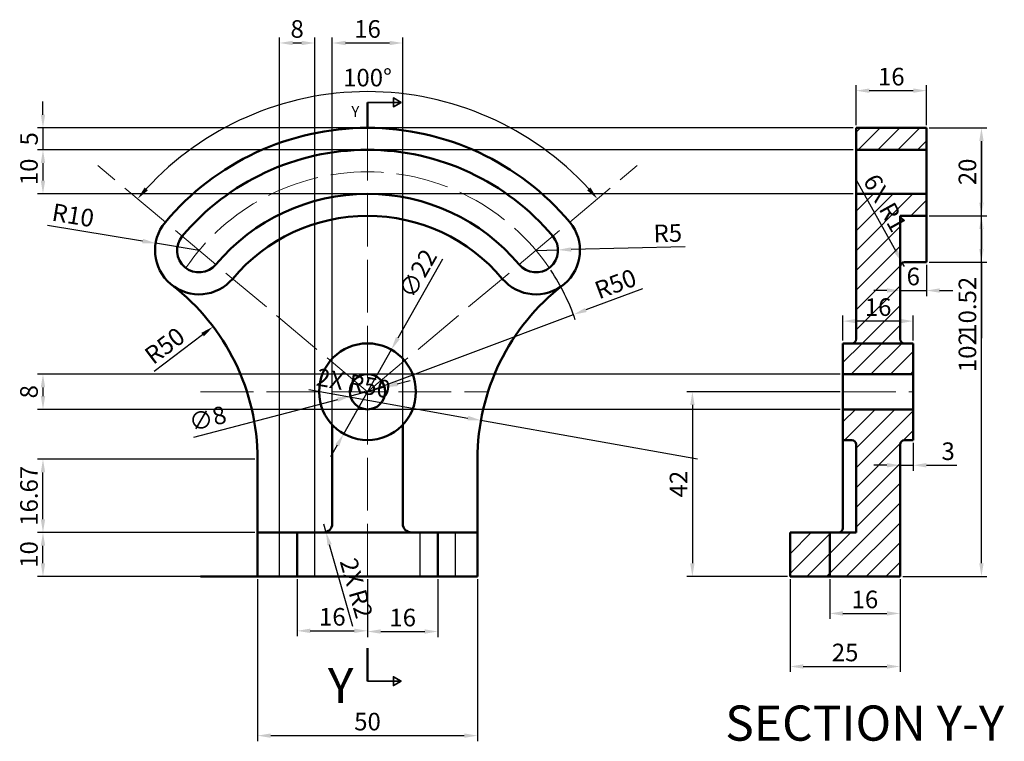
# Model space of a CAD drawing. Units: millimetres. Extents: x 867 to 1199, y -58 to 305.
# Tile 3 of 3: x 867 to 1091, y 141 to 305. Entities that reach past the tile are written whole.
import ezdxf

# ---------------------------------------------------------------- set-up
doc = ezdxf.new("R2010")
doc.units = ezdxf.units.MM
doc.linetypes.add('ACAD_ISO02W100', pattern=[15, 12, -3])
for name, color, linetype, lineweight in [('M-CNTR', 1, 'ACAD_ISO02W100', 18), ('M-DIMS', 2, 'Continuous', 25), ('M-HATC', 8, 'Continuous', 18), ('M-HIDN', 6, 'ACAD_ISO02W100', 25), ('M-OUTL', 7, 'Continuous', 50), ('M-SECT', 4, 'Continuous', 35), ('M-TEXT', 3, 'Continuous', 25)]:
    doc.layers.add(name, color=color, linetype=linetype, lineweight=lineweight)
doc.styles.get("Standard").update_dxf_attribs({"font": 'arial.ttf'})
doc.dimstyles.new('ISO-25', dxfattribs={"dimtxt": 4, "dimasz": 3, "dimexe": 1.25, "dimexo": 0.625, "dimtad": 1, "dimdec": 1, "dimtxsty": 'Standard', "dimcen": 2.5, "dimadec": 0, "dimazin": 0, "dimtfac": 1, "dimtdec": 1, "dimtmove": 0, "dimatfit": 3, "dimfxl": 1, "dimarcsym": 0})
pattern_1 = [(45, (-91.2894, -451.28), (-2.245064, 2.245064), [])]

# ---------------------------------------------------------------- blocks, each defined once
blk = doc.blocks.new('*D1')
at = {"layer": 'Defpoints', "color": 0, "transparency": 16777216}
for p in [(921.2, 178.7), (971.2, 178.7), (971.2, 142.51)]:
    blk.add_point(p, dxfattribs=at)
at = {"layer": 'M-DIMS', "color": 0, "lineweight": -2, "transparency": 16777216}
for p, q in [((921.2, 178.08), (921.2, 141.26)), ((971.2, 178.08), (971.2, 141.26)), ((924.2, 142.51), (968.2, 142.51))]:
    blk.add_line(p, q, dxfattribs=at)
at = {"layer": 'M-DIMS', "color": 0, "transparency": 16777216}
for points in [[(924.2, 143.01), (924.2, 142.01), (921.2, 142.51)], [(968.2, 143.01), (968.2, 142.01), (971.2, 142.51)]]:
    blk.add_solid(points, dxfattribs=at)
at = {"layer": 'M-DIMS', "color": 0, "transparency": 16777216, "insert": (946.2, 145.18), "char_height": 4, "attachment_point": 5}
blk.add_mtext('50', dxfattribs=at)
blk = doc.blocks.new('*D2')
at = {"layer": 'Defpoints', "color": 0, "transparency": 16777216}
for p in [(930.2, 178.7), (946.2, 178.7), (946.2, 166.34)]:
    blk.add_point(p, dxfattribs=at)
at = {"layer": 'M-DIMS', "color": 0, "lineweight": -2, "transparency": 16777216}
for p, q in [((930.2, 178.08), (930.2, 165.09)), ((946.2, 178.08), (946.2, 165.09)), ((933.2, 166.34), (943.2, 166.34))]:
    blk.add_line(p, q, dxfattribs=at)
at = {"layer": 'M-DIMS', "color": 0, "transparency": 16777216}
for points in [[(933.2, 166.84), (933.2, 165.84), (930.2, 166.34)], [(943.2, 166.84), (943.2, 165.84), (946.2, 166.34)]]:
    blk.add_solid(points, dxfattribs=at)
at = {"layer": 'M-DIMS', "color": 0, "transparency": 16777216, "insert": (938.2, 169.01), "char_height": 4, "attachment_point": 5}
blk.add_mtext('16', dxfattribs=at)
blk = doc.blocks.new('*D3')
at = {"layer": 'Defpoints', "color": 0, "transparency": 16777216}
for p in [(946.2, 178.7), (962.2, 178.7), (962.2, 166.18)]:
    blk.add_point(p, dxfattribs=at)
at = {"layer": 'M-DIMS', "color": 0, "lineweight": -2, "transparency": 16777216}
for p, q in [((946.2, 178.08), (946.2, 164.93)), ((962.2, 178.08), (962.2, 164.93)), ((949.2, 166.18), (959.2, 166.18))]:
    blk.add_line(p, q, dxfattribs=at)
at = {"layer": 'M-DIMS', "color": 0, "transparency": 16777216}
for points in [[(949.2, 166.68), (949.2, 165.68), (946.2, 166.18)], [(959.2, 166.68), (959.2, 165.68), (962.2, 166.18)]]:
    blk.add_solid(points, dxfattribs=at)
at = {"layer": 'M-DIMS', "color": 0, "transparency": 16777216, "insert": (954.2, 168.84), "char_height": 4, "attachment_point": 5}
blk.add_mtext('16', dxfattribs=at)
blk = doc.blocks.new('*D4')
at = {"layer": 'Defpoints', "color": 0, "transparency": 16777216}
for p in [(898.03, 254.48), (907.9, 252.84)]:
    blk.add_point(p, dxfattribs=at)
at = {"layer": 'M-DIMS', "color": 0, "lineweight": -2, "transparency": 16777216}
for p, q in [((873.42, 258.58), (895.07, 254.98)), ((907.9, 252.84), (898.03, 254.48))]:
    blk.add_line(p, q, dxfattribs=at)
at = {"layer": 'M-DIMS', "color": 0, "transparency": 16777216}
blk.add_solid([(895.16, 255.47), (894.99, 254.48), (898.03, 254.48)], dxfattribs=at)
at = {"layer": 'M-DIMS', "color": 0, "transparency": 16777216, "insert": (879.18, 260.33), "char_height": 4, "attachment_point": 5, "rotation": 350.5421}
blk.add_mtext('R10', dxfattribs=at)
blk = doc.blocks.new('*D5')
at = {"layer": 'Defpoints', "color": 0, "transparency": 16777216}
for p in [(989.5, 252.96), (984.5, 252.84)]:
    blk.add_point(p, dxfattribs=at)
at = {"layer": 'M-DIMS', "color": 0, "lineweight": -2, "transparency": 16777216}
for p, q in [((984.5, 252.84), (989.5, 252.96)), ((1018.41, 253.67), (992.5, 253.04))]:
    blk.add_line(p, q, dxfattribs=at)
at = {"layer": 'M-DIMS', "color": 0, "transparency": 16777216}
blk.add_solid([(992.49, 253.54), (992.51, 252.54), (989.5, 252.96)], dxfattribs=at)
at = {"layer": 'M-DIMS', "color": 0, "transparency": 16777216, "insert": (1014.48, 256.24), "char_height": 4, "attachment_point": 5, "rotation": 1.4057}
blk.add_mtext('R5', dxfattribs=at)
blk = doc.blocks.new('*D6')
at = {"layer": 'Defpoints', "color": 0, "transparency": 16777216}
for p in [(993.02, 238.24), (946.2, 220.7)]:
    blk.add_point(p, dxfattribs=at)
at = {"layer": 'M-DIMS', "color": 0, "lineweight": -2, "transparency": 16777216}
for p, q in [((1008.75, 244.13), (995.83, 239.29)), ((946.2, 220.7), (993.02, 238.24))]:
    blk.add_line(p, q, dxfattribs=at)
blk.add_arc((946.2, 220.7), 50, 19.1042, 33.5518, dxfattribs=at)
at = {"layer": 'M-DIMS', "color": 0, "transparency": 16777216}
blk.add_solid([(995.66, 239.76), (996.01, 238.82), (993.02, 238.24)], dxfattribs=at)
at = {"layer": 'M-DIMS', "color": 0, "transparency": 16777216, "insert": (1002.76, 244.74), "char_height": 4, "attachment_point": 5, "rotation": 20.5366}
blk.add_mtext('R50', dxfattribs=at)
blk = doc.blocks.new('*D7')
at = {"layer": 'Defpoints', "color": 0, "transparency": 16777216}
for p in [(911.1, 235.5), (871.2, 205.37)]:
    blk.add_point(p, dxfattribs=at)
at = {"layer": 'M-DIMS', "color": 0, "lineweight": -2, "transparency": 16777216}
blk.add_line((897.7, 225.38), (908.71, 233.69), dxfattribs=at)
at = {"layer": 'M-DIMS', "color": 0, "transparency": 16777216}
blk.add_solid([(908.41, 234.09), (909.01, 233.29), (911.1, 235.5)], dxfattribs=at)
at = {"layer": 'M-DIMS', "color": 0, "transparency": 16777216, "insert": (900.4, 230.76), "char_height": 4, "attachment_point": 5, "rotation": 37.0544}
blk.add_mtext('R50', dxfattribs=at)
blk = doc.blocks.new('*D8')
at = {"layer": 'Defpoints', "color": 0, "transparency": 16777216}
for p in [(951.62, 230.27), (940.78, 211.13)]:
    blk.add_point(p, dxfattribs=at)
at = {"layer": 'M-DIMS', "color": 0, "lineweight": -2, "transparency": 16777216}
for p, q in [((963.28, 250.87), (953.1, 232.88)), ((940.78, 211.13), (951.62, 230.27)), ((939.3, 208.52), (937.82, 205.91))]:
    blk.add_line(p, q, dxfattribs=at)
at = {"layer": 'M-DIMS', "color": 0, "transparency": 16777216}
for points in [[(952.66, 233.13), (953.53, 232.64), (951.62, 230.27)], [(938.87, 208.76), (939.74, 208.27), (940.78, 211.13)]]:
    blk.add_solid(points, dxfattribs=at)
at = {"layer": 'M-DIMS', "color": 0, "transparency": 16777216, "insert": (958.08, 247.33), "char_height": 4, "attachment_point": 5, "rotation": 60.4785}
blk.add_mtext('∅22', dxfattribs=at)
blk = doc.blocks.new('*D9')
at = {"layer": 'Defpoints', "color": 0, "transparency": 16777216}
for p in [(950.07, 221.71), (942.33, 219.69)]:
    blk.add_point(p, dxfattribs=at)
at = {"layer": 'M-DIMS', "color": 0, "lineweight": -2, "transparency": 16777216}
for p, q in [((950.07, 221.71), (942.33, 219.69)), ((952.97, 222.47), (955.87, 223.23)), ((906.7, 210.39), (939.43, 218.93))]:
    blk.add_line(p, q, dxfattribs=at)
at = {"layer": 'M-DIMS', "color": 0, "transparency": 16777216}
for points in [[(952.85, 222.95), (953.1, 221.99), (950.07, 221.71)], [(939.3, 219.42), (939.55, 218.45), (942.33, 219.69)]]:
    blk.add_solid(points, dxfattribs=at)
at = {"layer": 'M-DIMS', "color": 0, "transparency": 16777216, "insert": (909.98, 214.12), "char_height": 4, "attachment_point": 5, "rotation": 14.6342}
blk.add_mtext('∅8', dxfattribs=at)
blk = doc.blocks.new('*D10')
at = {"layer": 'Defpoints', "color": 0, "transparency": 16777216}
for p in [(965.77, 286.07), (884.92, 272.12), (1007.48, 272.12), (946.2, 220.7), (946.2, 220.7)]:
    blk.add_point(p, dxfattribs=at)
at = {"layer": 'M-DIMS', "color": 0, "lineweight": -2, "transparency": 16777216}
blk.add_arc((946.2, 220.7), 68.24, 42.5191, 137.4809, dxfattribs=at)
at = {"layer": 'M-DIMS', "color": 0, "transparency": 16777216}
for points in [[(896.28, 266.49), (895.53, 267.15), (893.93, 264.56)], [(996.87, 267.15), (996.12, 266.49), (998.47, 264.56)]]:
    blk.add_solid(points, dxfattribs=at)
at = {"layer": 'M-DIMS', "color": 0, "transparency": 16777216, "insert": (946.2, 291.61), "char_height": 4, "attachment_point": 5}
blk.add_mtext('100°', dxfattribs=at)
blk = doc.blocks.new('*D11')
at = {"layer": 'Defpoints', "color": 0, "transparency": 16777216}
for p in [(1073.28, 289.16), (1057.28, 280.7), (1073.28, 280.7)]:
    blk.add_point(p, dxfattribs=at)
at = {"layer": 'M-DIMS', "color": 0, "lineweight": -2, "transparency": 16777216}
for p, q in [((1057.28, 281.33), (1057.28, 290.41)), ((1060.28, 289.16), (1070.28, 289.16)), ((1073.28, 281.33), (1073.28, 290.41))]:
    blk.add_line(p, q, dxfattribs=at)
at = {"layer": 'M-DIMS', "color": 0, "transparency": 16777216}
for points in [[(1060.28, 289.66), (1060.28, 288.66), (1057.28, 289.16)], [(1070.28, 289.66), (1070.28, 288.66), (1073.28, 289.16)]]:
    blk.add_solid(points, dxfattribs=at)
at = {"layer": 'M-DIMS', "color": 0, "transparency": 16777216, "insert": (1065.28, 291.83), "char_height": 4, "attachment_point": 5}
blk.add_mtext('16', dxfattribs=at)
blk = doc.blocks.new('*D12')
at = {"layer": 'Defpoints', "color": 0, "transparency": 16777216}
for p in [(1073.28, 250.18), (1067.28, 246.7), (1073.28, 243.72)]:
    blk.add_point(p, dxfattribs=at)
at = {"layer": 'M-DIMS', "color": 0, "lineweight": -2, "transparency": 16777216}
for p, q in [((1073.28, 249.56), (1073.28, 242.47)), ((1067.28, 246.08), (1067.28, 242.47)), ((1064.28, 243.72), (1061.28, 243.72)), ((1067.28, 243.72), (1073.28, 243.72)), ((1076.28, 243.72), (1079.28, 243.72))]:
    blk.add_line(p, q, dxfattribs=at)
at = {"layer": 'M-DIMS', "color": 0, "transparency": 16777216}
for points in [[(1064.28, 244.22), (1064.28, 243.22), (1067.28, 243.72)], [(1076.28, 244.22), (1076.28, 243.22), (1073.28, 243.72)]]:
    blk.add_solid(points, dxfattribs=at)
at = {"layer": 'M-DIMS', "color": 0, "transparency": 16777216, "insert": (1070.28, 246.39), "char_height": 4, "attachment_point": 5}
blk.add_mtext('6', dxfattribs=at)
blk = doc.blocks.new('*D13')
at = {"layer": 'Defpoints', "color": 0, "transparency": 16777216}
for p in [(1054.28, 236.76), (1054.28, 231.7), (1070.28, 231.7)]:
    blk.add_point(p, dxfattribs=at)
at = {"layer": 'M-DIMS', "color": 0, "lineweight": -2, "transparency": 16777216}
for p, q in [((1054.28, 232.33), (1054.28, 238.01)), ((1070.28, 232.33), (1070.28, 238.01)), ((1067.28, 236.76), (1057.28, 236.76))]:
    blk.add_line(p, q, dxfattribs=at)
at = {"layer": 'M-DIMS', "color": 0, "transparency": 16777216}
for points in [[(1057.28, 237.26), (1057.28, 236.26), (1054.28, 236.76)], [(1067.28, 237.26), (1067.28, 236.26), (1070.28, 236.76)]]:
    blk.add_solid(points, dxfattribs=at)
at = {"layer": 'M-DIMS', "color": 0, "transparency": 16777216, "insert": (1062.28, 239.43), "char_height": 4, "attachment_point": 5}
blk.add_mtext('16', dxfattribs=at)
blk = doc.blocks.new('*D14')
at = {"layer": 'Defpoints', "color": 0, "transparency": 16777216}
for p in [(1054.28, 220.7), (1020.06, 178.7), (1042.28, 178.7)]:
    blk.add_point(p, dxfattribs=at)
at = {"layer": 'M-DIMS', "color": 0, "lineweight": -2, "transparency": 16777216}
for p, q in [((1053.65, 220.7), (1018.81, 220.7)), ((1020.06, 217.7), (1020.06, 181.7)), ((1041.65, 178.7), (1018.81, 178.7))]:
    blk.add_line(p, q, dxfattribs=at)
at = {"layer": 'M-DIMS', "color": 0, "transparency": 16777216}
for points in [[(1019.56, 217.7), (1020.56, 217.7), (1020.06, 220.7)], [(1019.56, 181.7), (1020.56, 181.7), (1020.06, 178.7)]]:
    blk.add_solid(points, dxfattribs=at)
at = {"layer": 'M-DIMS', "color": 0, "transparency": 16777216, "insert": (1017.43, 199.7), "char_height": 4, "attachment_point": 5, "rotation": 90}
blk.add_mtext('42', dxfattribs=at)
blk = doc.blocks.new('*D15')
at = {"layer": 'Defpoints', "color": 0, "transparency": 16777216}
for p in [(1042.28, 178.7), (1067.28, 178.7), (1067.28, 158.23)]:
    blk.add_point(p, dxfattribs=at)
at = {"layer": 'M-DIMS', "color": 0, "lineweight": -2, "transparency": 16777216}
for p, q in [((1042.28, 178.08), (1042.28, 156.98)), ((1067.28, 178.08), (1067.28, 156.98)), ((1045.28, 158.23), (1064.28, 158.23))]:
    blk.add_line(p, q, dxfattribs=at)
at = {"layer": 'M-DIMS', "color": 0, "transparency": 16777216}
for points in [[(1045.28, 158.73), (1045.28, 157.73), (1042.28, 158.23)], [(1064.28, 158.73), (1064.28, 157.73), (1067.28, 158.23)]]:
    blk.add_solid(points, dxfattribs=at)
at = {"layer": 'M-DIMS', "color": 0, "transparency": 16777216, "insert": (1054.78, 160.9), "char_height": 4, "attachment_point": 5}
blk.add_mtext('25', dxfattribs=at)
blk = doc.blocks.new('*D16')
at = {"layer": 'Defpoints', "color": 0, "transparency": 16777216}
for p in [(1051.28, 178.7), (1067.28, 178.7), (1067.28, 170.29)]:
    blk.add_point(p, dxfattribs=at)
at = {"layer": 'M-DIMS', "color": 0, "lineweight": -2, "transparency": 16777216}
for p, q in [((1051.28, 178.08), (1051.28, 169.04)), ((1067.28, 178.08), (1067.28, 169.04)), ((1054.28, 170.29), (1064.28, 170.29))]:
    blk.add_line(p, q, dxfattribs=at)
at = {"layer": 'M-DIMS', "color": 0, "transparency": 16777216}
for points in [[(1054.28, 170.79), (1054.28, 169.79), (1051.28, 170.29)], [(1064.28, 170.79), (1064.28, 169.79), (1067.28, 170.29)]]:
    blk.add_solid(points, dxfattribs=at)
at = {"layer": 'M-DIMS', "color": 0, "transparency": 16777216, "insert": (1059.28, 172.96), "char_height": 4, "attachment_point": 5}
blk.add_mtext('16', dxfattribs=at)
blk = doc.blocks.new('*D17')
at = {"layer": 'Defpoints', "color": 0, "transparency": 16777216}
for p in [(1070.28, 209.7), (1067.28, 206.36), (1070.28, 203.99)]:
    blk.add_point(p, dxfattribs=at)
at = {"layer": 'M-DIMS', "color": 0, "lineweight": -2, "transparency": 16777216}
for p, q in [((1070.28, 209.08), (1070.28, 202.74)), ((1064.28, 203.99), (1061.28, 203.99)), ((1067.28, 205.74), (1067.28, 202.74)), ((1067.28, 203.99), (1070.28, 203.99)), ((1073.28, 203.99), (1080.15, 203.99))]:
    blk.add_line(p, q, dxfattribs=at)
at = {"layer": 'M-DIMS', "color": 0, "transparency": 16777216}
for points in [[(1064.28, 204.49), (1064.28, 203.49), (1067.28, 203.99)], [(1073.28, 204.49), (1073.28, 203.49), (1070.28, 203.99)]]:
    blk.add_solid(points, dxfattribs=at)
at = {"layer": 'M-DIMS', "color": 0, "transparency": 16777216, "insert": (1078.21, 206.66), "char_height": 4, "attachment_point": 5}
blk.add_mtext('3', dxfattribs=at)
blk = doc.blocks.new('*D47')
at = {"layer": 'Defpoints', "color": 0, "transparency": 16777216}
for p in [(934.2, 300), (926.2, 178.7), (934.2, 178.7)]:
    blk.add_point(p, dxfattribs=at)
at = {"layer": 'M-DIMS', "color": 0, "lineweight": -2, "transparency": 16777216}
for p, q in [((926.2, 179.33), (926.2, 301.25)), ((929.2, 300), (931.2, 300)), ((934.2, 179.33), (934.2, 301.25))]:
    blk.add_line(p, q, dxfattribs=at)
at = {"layer": 'M-DIMS', "color": 0, "transparency": 16777216}
for points in [[(929.2, 300.5), (929.2, 299.5), (926.2, 300)], [(931.2, 300.5), (931.2, 299.5), (934.2, 300)]]:
    blk.add_solid(points, dxfattribs=at)
at = {"layer": 'M-DIMS', "color": 0, "transparency": 16777216, "insert": (930.2, 302.67), "char_height": 4, "attachment_point": 5}
blk.add_mtext('8', dxfattribs=at)
blk = doc.blocks.new('*D48')
at = {"layer": 'Defpoints', "color": 0, "transparency": 16777216}
for p in [(954.2, 300), (938.2, 190.7), (954.2, 190.7)]:
    blk.add_point(p, dxfattribs=at)
at = {"layer": 'M-DIMS', "color": 0, "lineweight": -2, "transparency": 16777216}
for p, q in [((938.2, 191.33), (938.2, 301.25)), ((941.2, 300), (951.2, 300)), ((954.2, 191.33), (954.2, 301.25))]:
    blk.add_line(p, q, dxfattribs=at)
at = {"layer": 'M-DIMS', "color": 0, "transparency": 16777216}
for points in [[(941.2, 300.5), (941.2, 299.5), (938.2, 300)], [(951.2, 300.5), (951.2, 299.5), (954.2, 300)]]:
    blk.add_solid(points, dxfattribs=at)
at = {"layer": 'M-DIMS', "color": 0, "transparency": 16777216, "insert": (946.2, 302.67), "char_height": 4, "attachment_point": 5}
blk.add_mtext('16', dxfattribs=at)
blk = doc.blocks.new('*D49')
at = {"layer": 'Defpoints', "color": 0, "transparency": 16777216}
for p in [(872.42, 188.7), (921.2, 188.7), (921.2, 178.7)]:
    blk.add_point(p, dxfattribs=at)
at = {"layer": 'M-DIMS', "color": 0, "lineweight": -2, "transparency": 16777216}
for p, q in [((920.57, 188.7), (871.17, 188.7)), ((872.42, 181.7), (872.42, 185.7)), ((920.57, 178.7), (871.17, 178.7))]:
    blk.add_line(p, q, dxfattribs=at)
at = {"layer": 'M-DIMS', "color": 0, "transparency": 16777216}
for points in [[(871.92, 185.7), (872.92, 185.7), (872.42, 188.7)], [(871.92, 181.7), (872.92, 181.7), (872.42, 178.7)]]:
    blk.add_solid(points, dxfattribs=at)
at = {"layer": 'M-DIMS', "color": 0, "transparency": 16777216, "insert": (869.75, 183.7), "char_height": 4, "attachment_point": 5, "rotation": 90}
blk.add_mtext('10', dxfattribs=at)
blk = doc.blocks.new('*D50')
at = {"layer": 'Defpoints', "color": 0, "transparency": 16777216}
for p in [(872.42, 205.37), (921.2, 205.37), (921.2, 188.7)]:
    blk.add_point(p, dxfattribs=at)
at = {"layer": 'M-DIMS', "color": 0, "lineweight": -2, "transparency": 16777216}
for p, q in [((920.57, 205.37), (871.17, 205.37)), ((872.42, 191.7), (872.42, 202.37)), ((920.57, 188.7), (871.17, 188.7))]:
    blk.add_line(p, q, dxfattribs=at)
at = {"layer": 'M-DIMS', "color": 0, "transparency": 16777216}
for points in [[(871.92, 202.37), (872.92, 202.37), (872.42, 205.37)], [(871.92, 191.7), (872.92, 191.7), (872.42, 188.7)]]:
    blk.add_solid(points, dxfattribs=at)
at = {"layer": 'M-DIMS', "color": 0, "transparency": 16777216, "insert": (869.75, 197.04), "char_height": 4, "attachment_point": 5, "rotation": 90}
blk.add_mtext('16.67', dxfattribs=at)
blk = doc.blocks.new('*D51')
at = {"layer": 'Defpoints', "color": 0, "transparency": 16777216}
for p in [(1073.28, 280.7), (1085.78, 280.7), (1067.28, 178.7)]:
    blk.add_point(p, dxfattribs=at)
at = {"layer": 'M-DIMS', "color": 0, "lineweight": -2, "transparency": 16777216}
for p, q in [((1073.9, 280.7), (1087.03, 280.7)), ((1085.78, 181.7), (1085.78, 277.7)), ((1067.9, 178.7), (1087.03, 178.7))]:
    blk.add_line(p, q, dxfattribs=at)
at = {"layer": 'M-DIMS', "color": 0, "transparency": 16777216}
for points in [[(1085.28, 277.7), (1086.28, 277.7), (1085.78, 280.7)], [(1085.28, 181.7), (1086.28, 181.7), (1085.78, 178.7)]]:
    blk.add_solid(points, dxfattribs=at)
at = {"layer": 'M-DIMS', "color": 0, "transparency": 16777216, "insert": (1083.11, 229.7), "char_height": 4, "attachment_point": 5, "rotation": 90}
blk.add_mtext('102', dxfattribs=at)
blk = doc.blocks.new('*D52')
at = {"layer": 'Defpoints', "color": 0, "transparency": 16777216}
for p in [(1073.28, 280.7), (1073.28, 260.7), (1085.78, 260.7)]:
    blk.add_point(p, dxfattribs=at)
at = {"layer": 'M-DIMS', "color": 0, "lineweight": -2, "transparency": 16777216}
for p, q in [((1073.9, 280.7), (1087.03, 280.7)), ((1085.78, 277.7), (1085.78, 263.7)), ((1073.9, 260.7), (1087.03, 260.7))]:
    blk.add_line(p, q, dxfattribs=at)
at = {"layer": 'M-DIMS', "color": 0, "transparency": 16777216}
for points in [[(1085.28, 277.7), (1086.28, 277.7), (1085.78, 280.7)], [(1085.28, 263.7), (1086.28, 263.7), (1085.78, 260.7)]]:
    blk.add_solid(points, dxfattribs=at)
at = {"layer": 'M-DIMS', "color": 0, "transparency": 16777216, "insert": (1083.11, 270.7), "char_height": 4, "attachment_point": 5, "rotation": 90}
blk.add_mtext('20', dxfattribs=at)
blk = doc.blocks.new('*D53')
at = {"layer": 'Defpoints', "color": 0, "transparency": 16777216}
for p in [(1073.28, 260.7), (1073.28, 250.18), (1085.78, 250.18)]:
    blk.add_point(p, dxfattribs=at)
at = {"layer": 'M-DIMS', "color": 0, "lineweight": -2, "transparency": 16777216}
for p, q in [((1073.9, 260.7), (1087.03, 260.7)), ((1085.78, 257.7), (1085.78, 253.18)), ((1073.9, 250.18), (1087.03, 250.18)), ((1085.78, 250.18), (1085.78, 232.85))]:
    blk.add_line(p, q, dxfattribs=at)
at = {"layer": 'M-DIMS', "color": 0, "transparency": 16777216}
for points in [[(1085.28, 257.7), (1086.28, 257.7), (1085.78, 260.7)], [(1085.28, 253.18), (1086.28, 253.18), (1085.78, 250.18)]]:
    blk.add_solid(points, dxfattribs=at)
at = {"layer": 'M-DIMS', "color": 0, "transparency": 16777216, "insert": (1083.11, 240.02), "char_height": 4, "attachment_point": 5, "rotation": 90}
blk.add_mtext('10.52', dxfattribs=at)
blk = doc.blocks.new('*D54')
at = {"layer": 'Defpoints', "color": 0, "transparency": 16777216}
for p in [(1057.28, 280.7), (872.42, 275.7), (1057.28, 275.7)]:
    blk.add_point(p, dxfattribs=at)
at = {"layer": 'M-DIMS', "color": 0, "lineweight": -2, "transparency": 16777216}
for p, q in [((872.42, 283.7), (872.42, 286.7)), ((1056.65, 280.7), (871.17, 280.7)), ((872.42, 280.7), (872.42, 275.7)), ((1056.65, 275.7), (871.17, 275.7)), ((872.42, 272.7), (872.42, 269.7))]:
    blk.add_line(p, q, dxfattribs=at)
at = {"layer": 'M-DIMS', "color": 0, "transparency": 16777216}
for points in [[(871.92, 283.7), (872.92, 283.7), (872.42, 280.7)], [(871.92, 272.7), (872.92, 272.7), (872.42, 275.7)]]:
    blk.add_solid(points, dxfattribs=at)
at = {"layer": 'M-DIMS', "color": 0, "transparency": 16777216, "insert": (869.76, 278.2), "char_height": 4, "attachment_point": 5, "rotation": 90}
blk.add_mtext('5', dxfattribs=at)
blk = doc.blocks.new('*D55')
at = {"layer": 'Defpoints', "color": 0, "transparency": 16777216}
for p in [(1057.28, 275.7), (872.42, 265.7), (1057.28, 265.7)]:
    blk.add_point(p, dxfattribs=at)
at = {"layer": 'M-DIMS', "color": 0, "lineweight": -2, "transparency": 16777216}
for p, q in [((1056.65, 275.7), (871.17, 275.7)), ((872.42, 272.7), (872.42, 268.7)), ((1056.65, 265.7), (871.17, 265.7))]:
    blk.add_line(p, q, dxfattribs=at)
at = {"layer": 'M-DIMS', "color": 0, "transparency": 16777216}
for points in [[(871.92, 272.7), (872.92, 272.7), (872.42, 275.7)], [(871.92, 268.7), (872.92, 268.7), (872.42, 265.7)]]:
    blk.add_solid(points, dxfattribs=at)
at = {"layer": 'M-DIMS', "color": 0, "transparency": 16777216, "insert": (869.75, 270.7), "char_height": 4, "attachment_point": 5, "rotation": 90}
blk.add_mtext('10', dxfattribs=at)
blk = doc.blocks.new('*D56')
at = {"layer": 'Defpoints', "color": 0, "transparency": 16777216}
for p in [(1054.28, 224.7), (872.42, 216.7), (1054.28, 216.7)]:
    blk.add_point(p, dxfattribs=at)
at = {"layer": 'M-DIMS', "color": 0, "lineweight": -2, "transparency": 16777216}
for p, q in [((1053.65, 224.7), (871.17, 224.7)), ((872.42, 221.7), (872.42, 219.7)), ((1053.65, 216.7), (871.17, 216.7))]:
    blk.add_line(p, q, dxfattribs=at)
at = {"layer": 'M-DIMS', "color": 0, "transparency": 16777216}
for points in [[(871.92, 221.7), (872.92, 221.7), (872.42, 224.7)], [(871.92, 219.7), (872.92, 219.7), (872.42, 216.7)]]:
    blk.add_solid(points, dxfattribs=at)
at = {"layer": 'M-DIMS', "color": 0, "transparency": 16777216, "insert": (869.75, 220.7), "char_height": 4, "attachment_point": 5, "rotation": 90}
blk.add_mtext('8', dxfattribs=at)
blk = doc.blocks.new('*D62')
at = {"layer": 'Defpoints', "color": 0, "transparency": 16777216}
for p in [(971.99, 214.2), (1021.2, 205.37)]:
    blk.add_point(p, dxfattribs=at)
at = {"layer": 'M-DIMS', "color": 0, "lineweight": -2, "transparency": 16777216}
for p, q in [((932.88, 221.22), (969.03, 214.73)), ((1021.2, 205.37), (971.99, 214.2))]:
    blk.add_line(p, q, dxfattribs=at)
at = {"layer": 'M-DIMS', "color": 0, "transparency": 16777216}
blk.add_solid([(969.12, 215.22), (968.94, 214.24), (971.99, 214.2)], dxfattribs=at)
at = {"layer": 'M-DIMS', "color": 0, "transparency": 16777216, "insert": (942.93, 222.13), "char_height": 4, "attachment_point": 5, "rotation": 349.8263}
blk.add_mtext('2X R50', dxfattribs=at)
blk = doc.blocks.new('*D63')
at = {"layer": 'Defpoints', "color": 0, "transparency": 16777216}
for p in [(936.2, 190.7), (936.75, 188.78)]:
    blk.add_point(p, dxfattribs=at)
at = {"layer": 'M-DIMS', "color": 0, "lineweight": -2, "transparency": 16777216}
for p, q in [((936.2, 190.7), (936.75, 188.78)), ((942.9, 167.32), (937.58, 185.89))]:
    blk.add_line(p, q, dxfattribs=at)
at = {"layer": 'M-DIMS', "color": 0, "transparency": 16777216}
blk.add_solid([(938.06, 186.03), (937.1, 185.76), (936.75, 188.78)], dxfattribs=at)
at = {"layer": 'M-DIMS', "color": 0, "transparency": 16777216, "insert": (943.18, 175.89), "char_height": 4, "attachment_point": 5, "rotation": 285.9851}
blk.add_mtext('2X R2', dxfattribs=at)
blk = doc.blocks.new('*D64')
at = {"layer": 'Defpoints', "color": 0, "transparency": 16777216}
for p in [(1067.79, 250.05), (1068.28, 249.18)]:
    blk.add_point(p, dxfattribs=at)
at = {"layer": 'M-DIMS', "color": 0, "lineweight": -2, "transparency": 16777216}
for p, q in [((1057.31, 268.88), (1066.33, 252.68)), ((1068.28, 249.18), (1067.79, 250.05))]:
    blk.add_line(p, q, dxfattribs=at)
at = {"layer": 'M-DIMS', "color": 0, "transparency": 16777216}
blk.add_solid([(1066.77, 252.92), (1065.9, 252.43), (1067.79, 250.05)], dxfattribs=at)
at = {"layer": 'M-DIMS', "color": 0, "transparency": 16777216, "insert": (1063.42, 263.38), "char_height": 4, "attachment_point": 5, "rotation": 299.1133}
blk.add_mtext('6X R1', dxfattribs=at)

msp = doc.modelspace()

# ---------------------------------------------------------------- hatches: boundary and pattern name
at = {"layer": 'M-HATC'}
h = msp.add_hatch(dxfattribs=at)
h.set_pattern_fill('ANSI31', color=256)
h.set_pattern_definition(pattern_1)
h.paths.add_polyline_path([(1073.279, 280.7), (1057.279, 280.7), (1057.279, 275.7), (1073.279, 275.7)])
h.paths.add_polyline_path([(1067.279, 260.7), (1073.279, 260.7), (1073.279, 265.7), (1057.279, 265.7), (1057.279, 231.7), (1067.279, 231.7)])
h = msp.add_hatch(dxfattribs=at)
h.set_pattern_fill('ANSI31', color=256)
h.set_pattern_definition(pattern_1)
h.paths.add_polyline_path([(1067.279, 208.7, -0.4142136), (1068.279, 209.7), (1070.279, 209.7), (1070.279, 216.7), (1054.279, 216.7), (1054.279, 209.7), (1056.279, 209.7, -0.4142136), (1057.279, 208.7), (1057.279, 188.7), (1051.279, 188.7), (1051.279, 178.7), (1067.279, 178.7)])
h.paths.add_polyline_path([(1070.279, 231.7), (1068.279, 231.7), (1054.279, 231.7), (1054.279, 224.7), (1070.279, 224.7)])
h.paths.add_polyline_path([(1051.279, 188.7), (1042.279, 188.7), (1042.279, 178.7), (1051.279, 178.7)])

# ---------------------------------------------------------------- linework, layer by layer
at = {"layer": 'M-CNTR'}
for p, q in [((946.199, 178.7), (946.199, 286.504)), ((946.199, 220.7), (884.915, 272.123)), ((946.199, 220.7), (1007.482, 272.123)), ((908.248, 220.7), (973.607, 220.7)), ((1054.279, 220.7), (1070.279, 220.7))]:
    msp.add_line(p, q, dxfattribs=at)
msp.add_arc((946.199, 220.7), 50, 34.26803, 145.73197, dxfattribs=at)
at = {"layer": 'M-HIDN'}
for p, q in [((926.199, 178.7), (926.199, 188.7)), ((934.199, 178.7), (934.199, 188.7)), ((958.199, 178.7), (958.199, 188.7)), ((966.199, 178.7), (966.199, 188.7))]:
    msp.add_line(p, q, dxfattribs=at)
at = {"layer": 'M-OUTL'}
for p, q in [((946.199, 280.7), (946.199, 286.504)), ((1057.279, 280.7), (1073.279, 280.7)), ((1057.279, 232.7), (1057.279, 280.7)), ((1073.279, 250.18), (1073.279, 280.7)), ((1057.279, 275.7), (1073.279, 275.7)), ((1057.279, 265.7), (1073.279, 265.7)), ((1067.279, 232.7), (1067.279, 260.7)), ((1067.279, 260.7), (1073.279, 260.7)), ((1073.279, 250.18), (1068.279, 250.18)), ((1054.279, 231.7), (1054.279, 209.7)), ((1054.279, 231.7), (1070.279, 231.7)), ((1056.279, 231.7), (1054.279, 231.7)), ((1070.279, 231.7), (1068.279, 231.7)), ((1070.279, 209.7), (1070.279, 231.7)), ((1054.279, 224.7), (1070.279, 224.7)), ((1054.279, 216.7), (1070.279, 216.7)), ((938.199, 190.7), (938.199, 213.151)), ((954.199, 190.7), (954.199, 213.151)), ((1054.279, 209.7), (1056.279, 209.7)), ((1054.279, 209.7), (1056.279, 209.7)), ((1054.279, 209.7), (1054.279, 189.7)), ((1057.279, 188.7), (1057.279, 208.7)), ((1067.279, 178.7), (1067.279, 208.7)), ((1068.279, 209.7), (1070.279, 209.7)), ((1068.279, 209.7), (1070.279, 209.7)), ((921.199, 178.7), (921.199, 205.371)), ((971.199, 178.7), (971.199, 205.371)), ((921.199, 188.7), (956.199, 188.7)), ((930.199, 178.7), (930.199, 188.7)), ((956.199, 188.7), (971.199, 188.7)), ((962.199, 178.7), (962.199, 188.7)), ((1042.279, 178.7), (1042.279, 188.7)), ((1042.279, 188.7), (1057.279, 188.7)), ((1051.279, 178.7), (1051.279, 188.7)), ((908.248, 178.7), (971.199, 178.7)), ((921.199, 178.7), (971.199, 178.7)), ((1042.279, 178.7), (1067.279, 178.7)), ((946.199, 154.896), (946.199, 162.427))]:
    msp.add_line(p, q, dxfattribs=at)
for radius in [11, 4]:
    msp.add_circle((946.199, 220.7), radius, dxfattribs=at)
for centre, radius, start, end in [((946.199, 220.7), 60, 40, 140), ((946.199, 220.7), 55, 40, 140), ((946.199, 220.7), 45, 40, 140), ((946.199, 220.7), 40, 40, 140), ((907.897, 252.84), 10, 140, 320), ((984.501, 252.84), 10, 220, 40), ((907.897, 252.84), 5, 140, 320), ((984.501, 252.84), 5, 220, 40), ((1068.279, 249.18), 1, 90, 180), ((871.199, 205.371), 50, 0, 52.29257), ((946.199, 220.7), 50, 151.47834, 151.50358), ((1021.199, 205.371), 50, 127.70743, 180), ((946.199, 220.7), 50, 28.49642, 28.52166), ((1056.279, 232.7), 1, 270, 0), ((1068.279, 232.7), 1, 180, 270), ((1056.279, 208.7), 1, 0, 90), ((1068.279, 208.7), 1, 90, 180), ((936.199, 190.7), 2, 270, 0), ((956.199, 190.7), 2, 180, 270), ((1053.279, 189.7), 1, 270, 0)]:
    msp.add_arc(centre, radius, start, end, dxfattribs=at)
at = {"layer": 'M-SECT'}
for points in [[(946.199, 286.504), (953.827, 286.504), (952.095, 287.504), (952.095, 286.504), (952.095, 285.504), (953.827, 286.504)], [(946.199, 154.896), (953.827, 154.896), (952.095, 153.896), (952.095, 154.896), (952.095, 155.896), (953.827, 154.896)]]:
    msp.add_lwpolyline(points, dxfattribs=at)

# ---------------------------------------------------------------- texts
at = {"layer": 'M-TEXT', "attachment_point": 1}
for s, insert, char_height in [('Y', (942.534, 285.665), 2.5), ('Y', (937.202, 157.9), 8), ('SECTION Y-Y', (1027.523, 149.362), 8)]:
    msp.add_mtext_dynamic_manual_height_columns(s, width=84.35545, gutter_width=12.5, heights=[0], dxfattribs=dict(at, insert=insert, char_height=char_height))

# ---------------------------------------------------------------- dimensions: what is measured, and where the dimension line sits
at = {"layer": 'M-DIMS'}
for base, p1, p2, override, picture, middle in [((934.199, 300.004), (926.199, 178.7), (934.199, 178.7), {"dimdec": 0, "dimlfac": 1, "dimrnd": 0, "dimzin": 0, "dimdsep": 46, "dimlunit": 2}, '*D47', (930.199, 302.672)), ((954.199, 300.004), (938.199, 190.7), (954.199, 190.7), {"dimdec": 0, "dimlfac": 1, "dimrnd": 0, "dimzin": 0, "dimdsep": 46, "dimlunit": 2}, '*D48', (946.199, 302.672)), ((1073.279, 289.161), (1057.279, 280.7), (1073.279, 280.7), {"dimclrd": 0, "dimclre": 0, "dimclrt": 0}, '*D11', (1065.279, 291.828)), ((1073.279, 243.723), (1067.279, 246.7), (1073.279, 250.18), {"dimclrd": 0, "dimclre": 0, "dimclrt": 0}, '*D12', (1070.279, 246.39)), ((1054.279, 236.761), (1070.279, 231.7), (1054.279, 231.7), {"dimclrd": 0, "dimclre": 0, "dimclrt": 0}, '*D13', (1062.279, 239.428)), ((1070.279, 203.988), (1067.279, 206.361), (1070.279, 209.7), {"dimclrd": 0, "dimclre": 0, "dimclrt": 0}, '*D17', (1078.214, 206.656)), ((971.199, 142.513), (921.199, 178.7), (971.199, 178.7), {"dimclrd": 0, "dimclre": 0, "dimclrt": 0}, '*D1', (946.199, 145.181)), ((946.199, 166.338), (930.199, 178.7), (946.199, 178.7), {"dimclrd": 0, "dimclre": 0, "dimclrt": 0}, '*D2', (938.199, 169.005)), ((962.199, 166.177), (946.199, 178.7), (962.199, 178.7), {"dimclrd": 0, "dimclre": 0, "dimclrt": 0}, '*D3', (954.199, 168.844)), ((1067.279, 158.232), (1042.279, 178.7), (1067.279, 178.7), {"dimclrd": 0, "dimclre": 0, "dimclrt": 0}, '*D15', (1054.779, 160.899)), ((1067.279, 170.291), (1051.279, 178.7), (1067.279, 178.7), {"dimclrd": 0, "dimclre": 0, "dimclrt": 0}, '*D16', (1059.279, 172.958))]:
    dim = msp.add_linear_dim(base=base, p1=p1, p2=p2, dimstyle='ISO-25', override=override, dxfattribs=at)
    dim.commit()
    dim.dimension.update_dxf_attribs({"geometry": picture, "text_midpoint": middle})
dim = msp.add_angular_dim_2l(base=(965.77, 286.072), line1=((946.199, 220.7), (1007.482, 272.123)), line2=((946.199, 220.7), (884.915, 272.123)), dimstyle='ISO-25', override={"dimclrd": 0, "dimclre": 0, "dimclrt": 0}, dxfattribs=at)
dim.commit()
dim.dimension.update_dxf_attribs({"geometry": '*D10', "text_midpoint": (946.199, 291.606)})
for base, p1, p2, override, picture, middle in [((872.415, 275.7), (1057.279, 280.7), (1057.279, 275.7), {"dimdec": 0, "dimlfac": 1, "dimrnd": 0, "dimzin": 0, "dimdsep": 46, "dimlunit": 2}, '*D54', (869.756, 278.2)), ((1085.779, 280.7), (1067.279, 178.7), (1073.279, 280.7), {"dimdec": 0, "dimlfac": 1, "dimrnd": 0, "dimzin": 0, "dimdsep": 46, "dimlunit": 2}, '*D51', (1083.112, 229.7)), ((1085.779, 260.7), (1073.279, 280.7), (1073.279, 260.7), {"dimdec": 0, "dimlfac": 1, "dimrnd": 0, "dimzin": 0, "dimdsep": 46, "dimlunit": 2}, '*D52', (1083.112, 270.7)), ((872.415, 265.7), (1057.279, 275.7), (1057.279, 265.7), {"dimdec": 0, "dimlfac": 1, "dimrnd": 0, "dimzin": 0, "dimdsep": 46, "dimlunit": 2}, '*D55', (869.748, 270.7)), ((1085.779, 250.18), (1073.279, 260.7), (1073.279, 250.18), {"dimdec": 2, "dimlfac": 1, "dimrnd": 0, "dimzin": 0, "dimdsep": 46, "dimlunit": 2}, '*D53', (1083.112, 240.015)), ((872.415, 216.7), (1054.279, 224.7), (1054.279, 216.7), {"dimdec": 0, "dimlfac": 1, "dimrnd": 0, "dimzin": 0, "dimdsep": 46, "dimlunit": 2}, '*D56', (869.748, 220.7)), ((1020.06, 178.7), (1054.279, 220.7), (1042.279, 178.7), {"dimclrd": 0, "dimclre": 0, "dimclrt": 0}, '*D14', (1017.427, 199.7)), ((872.415, 205.371), (921.199, 188.7), (921.199, 205.371), {"dimdec": 2, "dimlfac": 1, "dimrnd": 0, "dimzin": 0, "dimdsep": 46, "dimlunit": 2}, '*D50', (869.748, 197.036)), ((872.415, 188.7), (921.199, 178.7), (921.199, 188.7), {"dimdec": 0, "dimlfac": 1, "dimrnd": 0, "dimzin": 0, "dimdsep": 46, "dimlunit": 2}, '*D49', (869.748, 183.7))]:
    dim = msp.add_linear_dim(base=base, p1=p1, p2=p2, angle=90, dimstyle='ISO-25', override=override, dxfattribs=at)
    dim.commit()
    dim.dimension.update_dxf_attribs({"geometry": picture, "text_midpoint": middle})
for center, mpoint, text, picture, middle in [((1068.279, 249.18), (1067.793, 250.054), '6X <>', '*D64', (1063.422, 263.384)), ((936.199, 190.7), (936.75, 188.778), '2X <>', '*D63', (943.182, 175.89))]:
    dim = msp.add_radius_dim(center=center, mpoint=mpoint, text=text, dimstyle='ISO-25', override={"dimdec": 0, "dimlfac": 1, "dimrnd": 0, "dimzin": 0, "dimdsep": 46, "dimlunit": 2}, dxfattribs=at)
    dim.commit()
    dim.dimension.update_dxf_attribs({"geometry": picture, "text_midpoint": middle})
for center, mpoint, picture, middle in [((907.897, 252.84), (898.033, 254.483), '*D4', (878.741, 257.697)), ((984.501, 252.84), (989.5, 252.962), '*D5', (1014.548, 253.577)), ((871.199, 205.371), (911.102, 235.5), '*D7', (902.006, 228.632))]:
    dim = msp.add_radius_dim(center=center, mpoint=mpoint, dimstyle='ISO-25', override={"dimclrd": 0, "dimclre": 0, "dimclrt": 0}, dxfattribs=at)
    dim.commit()
    dim.dimension.update_dxf_attribs({"geometry": picture, "text_midpoint": middle, "dimtype": 164})
for p1, p2, picture, middle in [((940.779, 211.128), (951.619, 230.272), '*D8', (960.503, 245.961)), ((950.069, 221.711), (942.329, 219.69), '*D9', (910.686, 211.427))]:
    dim = msp.add_diameter_dim_2p(p1=p1, p2=p2, dimstyle='ISO-25', override={"dimclrd": 0, "dimclre": 0, "dimclrt": 0}, dxfattribs=at)
    dim.commit()
    dim.dimension.update_dxf_attribs({"geometry": picture, "text_midpoint": middle, "dimtype": 163})
dim = msp.add_radius_dim(center=(946.199, 220.7), mpoint=(993.021, 238.241), dimstyle='ISO-25', override={"dimclrd": 0, "dimclre": 0, "dimclrt": 0}, dxfattribs=at)
dim.commit()
dim.dimension.update_dxf_attribs({"geometry": '*D6', "text_midpoint": (1002.758, 244.737)})
dim = msp.add_radius_dim(center=(1021.199, 205.371), mpoint=(971.985, 214.203), text='2X <>', dimstyle='ISO-25', override={"dimdec": 0, "dimlfac": 1, "dimrnd": 0, "dimzin": 0, "dimdsep": 46, "dimlunit": 2}, dxfattribs=at)
dim.commit()
dim.dimension.update_dxf_attribs({"geometry": '*D62', "text_midpoint": (942.457, 219.502), "dimtype": 164})

doc.saveas('drawing.dxf')
